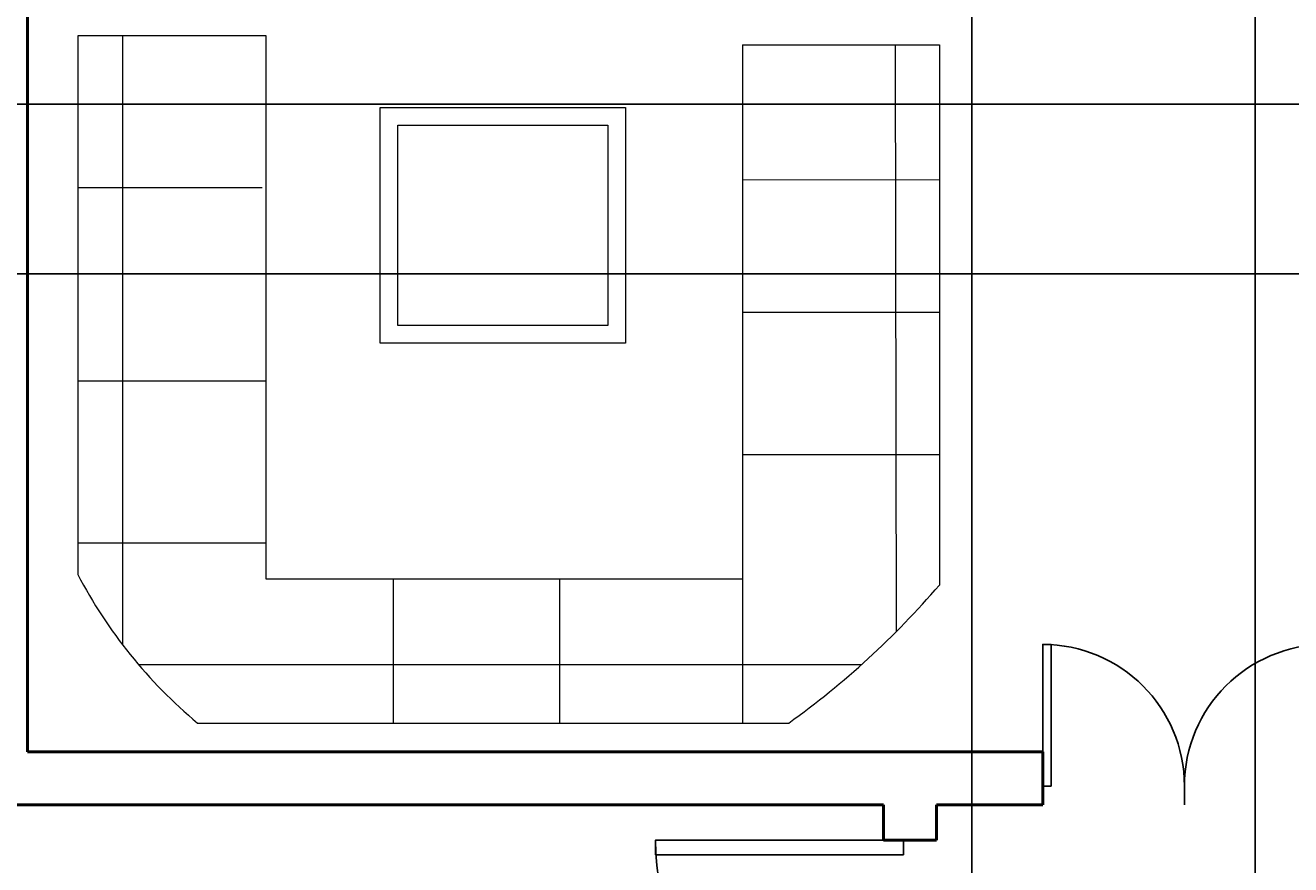
# Model space of a CAD drawing. Units: inches. Extents: x 5375 to 6084, y 16106 to 17259.
# Tile 22 of 32: x 5553 to 5768, y 16680 to 16823. Entities that reach past the tile are written whole.
import ezdxf

# ---------------------------------------------------------------- set-up
doc = ezdxf.new("R2010")
doc.units = ezdxf.units.IN
for name, color, linetype, lineweight in [('A-ANNO-DIMS', 2, 'Continuous', 18), ('DOOR', 4, 'Continuous', 25), ('FURNITURE', 3, 'Continuous', 18), ('WALL', 6, 'Continuous', 50)]:
    doc.layers.add(name, color=color, linetype=linetype, lineweight=lineweight)
doc.styles.get("Standard").update_dxf_attribs({"font": 'arial.ttf'})
doc.dimstyles.get("Standard").update_dxf_attribs({"dimtxt": 0.18, "dimasz": 0.18, "dimexe": 0.18, "dimexo": 0.0625, "dimgap": 0.09, "dimtad": 0, "dimtih": 1, "dimtoh": 1, "dimdec": 4, "dimzin": 0, "dimdsep": 46, "dimtxsty": 'Standard', "dimcen": 0.09, "dimadec": 0, "dimazin": 0, "dimtfac": 1, "dimtdec": 4, "dimtofl": 0, "dimtmove": 0, "dimatfit": 3, "dimfxl": 1, "dimtolj": 1, "dimtzin": 0, "dimarcsym": 0})

# ---------------------------------------------------------------- blocks, each defined once
blk = doc.blocks.new('*U2')
for p, q in [((0, 0), (0, -100)), ((750, 0), (750, -100))]:
    blk.add_line(p, q)
blk.add_lwpolyline([(0, 0), (0, 750), (43.75, 750), (43.75, 0)], close=True)
blk.add_arc((0, 0), 750, 0, 90)
blk = doc.blocks.new('*D39')
at = {"layer": 'A-ANNO-DIMS', "color": 0, "lineweight": -2, "transparency": 16777216}
for p, q in [((5713.62, 16402.64), (5713.62, 17259.16)), ((5713.8, 17258.98), (5737.4, 17258.98)), ((5761.44, 17258.98), (5737.84, 17258.98)), ((5761.62, 16402.64), (5761.62, 17259.16))]:
    blk.add_line(p, q, dxfattribs=at)
at = {"layer": 'A-ANNO-DIMS', "color": 0, "transparency": 16777216}
for points in [[(5713.8, 17259.01), (5713.8, 17258.95), (5713.62, 17258.98)], [(5761.44, 17259.01), (5761.44, 17258.95), (5761.62, 17258.98)]]:
    blk.add_solid(points, dxfattribs=at)
at = {"layer": 'Defpoints', "color": 0, "transparency": 16777216}
for p in [(5761.62, 17258.98), (5713.62, 16402.58), (5761.62, 16402.58)]:
    blk.add_point(p, dxfattribs=at)
at = {"layer": 'A-ANNO-DIMS', "color": 0, "transparency": 16777216, "insert": (5737.62, 17258.98), "char_height": 0.18, "attachment_point": 5}
blk.add_mtext('\\A1;48', dxfattribs=at)
blk = doc.blocks.new('*D43')
at = {"layer": 'A-ANNO-DIMS', "color": 0, "lineweight": -2, "transparency": 16777216}
for p, q in [((5826.06, 16809.37), (5375.56, 16809.37)), ((5375.74, 16809.19), (5375.74, 16795.15)), ((5375.74, 16780.76), (5375.74, 16794.79)), ((5826.06, 16780.58), (5375.56, 16780.58))]:
    blk.add_line(p, q, dxfattribs=at)
at = {"layer": 'A-ANNO-DIMS', "color": 0, "transparency": 16777216}
for points in [[(5375.71, 16809.19), (5375.77, 16809.19), (5375.74, 16809.37)], [(5375.71, 16780.76), (5375.77, 16780.76), (5375.74, 16780.58)]]:
    blk.add_solid(points, dxfattribs=at)
at = {"layer": 'Defpoints', "color": 0, "transparency": 16777216}
for p in [(5375.74, 16809.37), (5826.12, 16809.37), (5826.12, 16780.58)]:
    blk.add_point(p, dxfattribs=at)
at = {"layer": 'A-ANNO-DIMS', "color": 0, "transparency": 16777216, "insert": (5375.74, 16794.97), "char_height": 0.18, "attachment_point": 5}
blk.add_mtext('\\A1;28.786', dxfattribs=at)

msp = doc.modelspace()

# ---------------------------------------------------------------- linework, layer by layer
at = {"layer": 'FURNITURE'}
for p, q in [((5594.0817, 16820.9285), (5562.1447, 16820.9285)), ((5562.1447, 16820.9285), (5562.1447, 16729.6479)), ((5569.7561, 16820.9285), (5569.7561, 16717.6911)), ((5594.0685, 16728.8404), (5594.0685, 16820.9285)), ((5674.781, 16819.3936), (5708.1031, 16819.3936)), ((5674.781, 16819.3936), (5674.781, 16728.8404)), ((5700.6211, 16819.3936), (5700.7612, 16719.906)), ((5708.1031, 16819.3936), (5708.1031, 16727.8426)), ((5674.781, 16796.5293), (5708.1031, 16796.5763)), ((5593.4001, 16795.1755), (5562.1447, 16795.1755)), ((5674.781, 16774.117), (5708.1031, 16774.117)), ((5594.0685, 16762.3924), (5562.1447, 16762.3924)), ((5674.781, 16749.9584), (5708.1031, 16749.9584)), ((5594.0685, 16734.931), (5562.1447, 16734.931)), ((5674.781, 16728.8404), (5594.0685, 16728.8404)), ((5615.5782, 16728.8404), (5615.5782, 16704.4457)), ((5643.7766, 16728.8404), (5643.7766, 16704.4457)), ((5674.781, 16728.8404), (5674.781, 16704.4457)), ((5694.8688, 16714.3144), (5572.4804, 16714.3144)), ((5582.4391, 16704.4457), (5682.5927, 16704.4457))]:
    msp.add_line(p, q, dxfattribs=at)
for points in [[(5613.3867, 16808.8126), (5654.9275, 16808.8126), (5654.9275, 16768.8443), (5613.3867, 16768.8443)], [(5616.3802, 16805.8191), (5651.9339, 16805.8191), (5651.9339, 16771.8378), (5616.3802, 16771.8378)]]:
    msp.add_lwpolyline(points, close=True, dxfattribs=at)
for centre, radius, start, end in [((5635.4822, 16767.9318), 82.7288, 207.565606, 230.120973), ((5597.7253, 16822.5851), 145.4627, 305.692191, 319.35892)]:
    msp.add_arc(centre, radius, start, end, dxfattribs=at)
at = {"layer": 'WALL'}
for p, q in [((5553.6199, 16867.5793), (5553.6199, 16699.5793)), ((5553.6199, 16699.5793), (5725.6199, 16699.5793)), ((5725.6199, 16690.5793), (5725.6199, 16699.5793)), ((5536.6199, 16690.5793), (5698.6199, 16690.5793)), ((5698.6199, 16690.5793), (5698.6199, 16684.5793)), ((5707.6199, 16690.5793), (5707.6199, 16684.5793)), ((5707.6199, 16690.5793), (5725.6199, 16690.5793)), ((5707.6199, 16684.5793), (5698.6199, 16684.5793))]:
    msp.add_line(p, q, dxfattribs=at)

# ---------------------------------------------------------------- block references
at = {"layer": 'DOOR', "yscale": 0.0319999999999999, "zscale": 0.0319999999999999}
for p, xscale in [((5725.6199, 16693.7793), 0.0319999999999999), ((5773.6199, 16693.7793), -0.0319999999999999)]:
    msp.add_blockref('*U2', p, dxfattribs=dict(at, xscale=xscale))
at = {"layer": 'DOOR', "xscale": -0.0559999999999998, "yscale": 0.0559999999999998, "zscale": 0.0559999999999998, "rotation": 90}
msp.add_blockref('*U2', (5702.0199, 16684.5793), dxfattribs=at)

# ---------------------------------------------------------------- dimensions: what is measured, and where the dimension line sits
at = {"layer": 'A-ANNO-DIMS'}
dim = msp.add_linear_dim(base=(5761.6199, 17258.9793), p1=(5713.6199, 16402.5793), p2=(5761.6199, 16402.5793), dimstyle='Standard', override={"dimdec": 0, "dimlfac": 1, "dimrnd": 0, "dimzin": 0, "dimdsep": 46, "dimlunit": 2}, dxfattribs=at)
dim.commit()
dim.dimension.update_dxf_attribs({"geometry": '*D39', "text_midpoint": (5737.6199, 17258.9793)})
dim = msp.add_linear_dim(base=(5375.7423, 16809.3651), p1=(5826.1199, 16780.5793), p2=(5826.1199, 16809.3651), angle=90, dimstyle='Standard', override={"dimdec": 3, "dimlfac": 1, "dimrnd": 0, "dimzin": 0, "dimdsep": 46, "dimlunit": 2}, dxfattribs=at)
dim.commit()
dim.dimension.update_dxf_attribs({"geometry": '*D43', "text_midpoint": (5375.7423, 16794.9722)})

doc.saveas('drawing.dxf')
